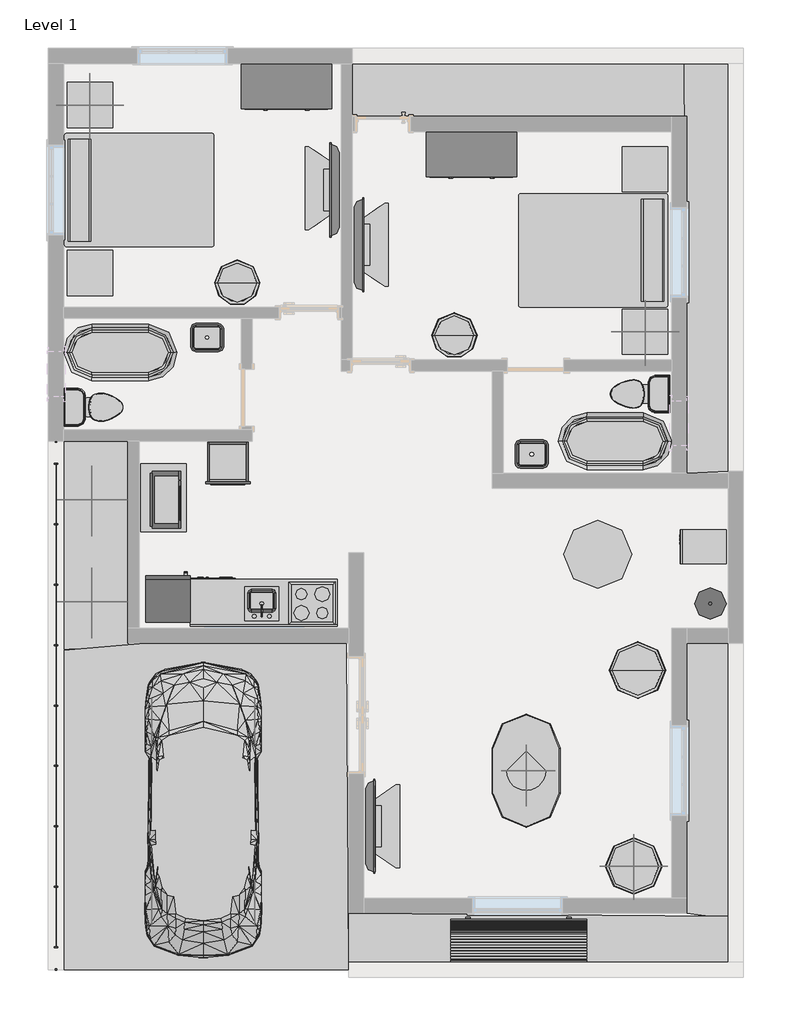
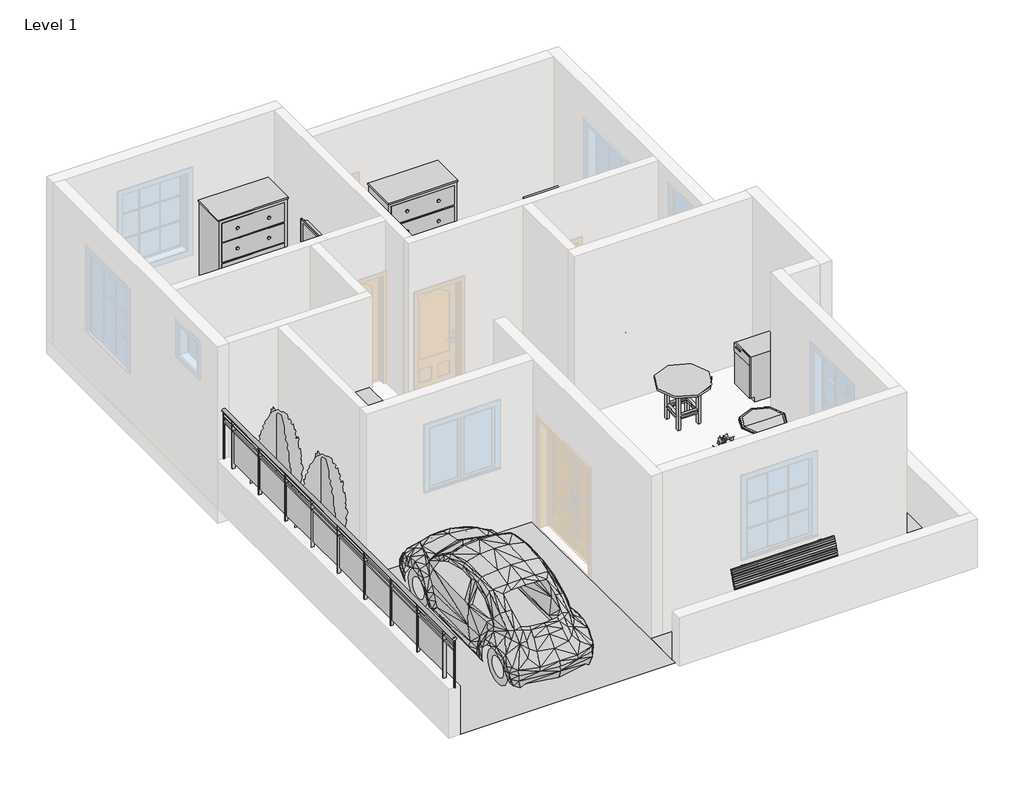
# One storey, part 2 of 2: 22 furniture elements, 14 proxies, 8 flow terminals, 7 geographic elements, 1 railing.
"""IFC4 building model written with IfcOpenShell, lengths in millimetres."""

from ifc_helpers import new_model, si_unit, point, frame, origin, place, context, project, spatial, polyline, ellipse_curve, trimmed, outline, extrude, triangles, transform, mapped, element, save
from ifc_brep_helpers import plane_surface, extruded_surface, advanced_brep
from components import proxy_7e1014cc, proxy_a6faaae8, proxy_45b28599, kitchenette_medium_kitchenette_medium_844211aa, proxy_8a8d5ab2, proxy_8b8c2dc4, rpc_beetle_rpc_beetle_3ce7ba48, proxy_c523a7b7, flow_terminal_871c2e40, flow_terminal_d49f872f, flow_terminal_62a433f7, toilet_domestic_3d_toilet_domestic_3d_f7549cf7, toilet_domestic_3d_toilet_domestic_3d_183bbd19, flow_terminal_b374fae2, furniture_e1791683, furniture_c6510c7c, furniture_9fa109b2, furniture_fdf74506, tv_stand_tv_stand_6ce107e5, furniture_582790c0, furniture_905aceb5, furniture_5bc9ed15, furniture_a672282c, table_round_2_a0cc3393, furniture_ebfaaaa6, geographic_element_235d1464, rpc_plant_tropical_55f6ff97, rpc_plant_tropical_agave_1_5_93a2a214, rpc_tree_conifer_chinese_juniper_7_1b9786cd

model = new_model("IFC4")

# Units and contexts
model_context = context("Model", 3, world=origin())
ifc_project = project(units=[si_unit("LENGTHUNIT", "METRE", prefix="MILLI")], contexts=[model_context])

# Site, building, storey
site = spatial("IfcSite", under=ifc_project)
building = spatial("IfcBuilding", under=site)
storey = spatial("IfcBuildingStorey", under=building, Name="Level 1", Elevation=0.0)

# Proxies
placement = place(None, origin())
element("IfcBuildingElementProxy", 1, Name="Building Element Proxy", at=placement, inside=storey, context=model_context, shape_type="Tessellation", body=[
    triangles([(-9901.0816956, 10267.8430298, 0.0), (-9037.4820831, 10267.8430298, 0.0), (-9037.4820831, 7550.0426422, 0.0), (-9901.0816956, 7550.0426422, 0.0), (-9901.0816956, 7466.0681168, 0.0), (-9032.7509766, 7492.9676376, 0.0), (-9033.9538101, 7484.1896851, 0.0)], [[7, 3, 5], [4, 5, 3], [1, 4, 3], [7, 6, 3], [3, 2, 1], [2, 3, 6]], closed=False),
])
element("IfcBuildingElementProxy", 2, Name="Building Element Proxy", at=placement, inside=storey, context=model_context, shape_type="Tessellation", body=[
    triangles([(-9901.0816956, 7456.8274017, 0.0), (-6098.1167313, 7550.0426422, 0.0), (-6072.0322769, 3155.8425453, 0.0), (-9901.0816956, 3155.8425453, 0.0), (-9026.5641449, 7481.0009262, 0.0), (-7567.2456619, 7524.6424484, 0.0), (-7984.5248428, 7517.1097687, 0.0), (-7982.6394928, 7524.6424484, 0.0), (-7985.2678207, 7537.342836, 0.0), (-8172.2232697, 7550.0426422, 0.0), (-8795.599173, 7550.0426422, 0.0), (-9021.7231613, 7526.2632797, 0.0)], [[4, 5, 1], [10, 5, 7], [1, 5, 12], [5, 11, 12], [11, 5, 10], [7, 9, 10], [12, 11, 1], [5, 4, 7], [8, 7, 6], [3, 7, 4], [6, 7, 3], [7, 8, 9], [6, 2, 10], [6, 9, 8], [2, 6, 3], [6, 10, 9]], closed=False),
])
element("IfcBuildingElementProxy", 3, Name="Building Element Proxy", at=placement, inside=storey, context=model_context, shape_type="Tessellation", body=[
    triangles([(-6065.6820831, 3917.8425453, 0.0), (-960.2821558, 3880.1032791, 0.0), (-960.2821558, 3257.4427391, 0.0), (-6065.6820831, 3257.4427391, 0.0)], [[1, 4, 2], [3, 2, 4]], closed=False),
])
element("IfcBuildingElementProxy", 4, Name="Building Element Proxy", at=placement, inside=storey, context=model_context, shape_type="Tessellation", body=[
    triangles([(-1519.0821316, 3917.8425453, 0.0), (-960.2821558, 3843.8738045, 0.0), (-1519.0821316, 7550.0426422, 0.0), (-960.2821558, 7550.0426422, 0.0)], [[3, 1, 4], [2, 4, 1]], closed=False),
])
element("IfcBuildingElementProxy", 5, Name="Building Element Proxy", at=placement, inside=storey, context=model_context, shape_type="Tessellation", body=[
    triangles([(-960.2821558, 9861.4422546, 0.0), (-1519.0821316, 9836.0426422, 0.0), (-1552.946925, 15347.8422546, 0.0), (-960.2821558, 15347.8422546, 0.0)], [[3, 2, 1], [1, 4, 3]], closed=False),
])
element("IfcBuildingElementProxy", 6, Name="Building Element Proxy", at=placement, inside=storey, context=model_context, shape_type="Tessellation", body=[
    triangles([(-1519.0821316, 14636.6426422, 0.0), (-1526.6161194, 15347.8422546, 0.0), (-6014.8822769, 15347.8422546, 0.0), (-6014.8822769, 14636.6426422, 0.0)], [[3, 4, 2], [1, 2, 4]], closed=False),
])
proxy_shape = proxy_7e1014cc(model_context)
element("IfcBuildingElementProxy", 7, Name="18\" x 24\" x 34 1/2\"", ObjectType="18\" x 24\" x 34 1/2\"", at=placement, inside=storey, context=model_context, shape_type="MappedRepresentation", body=[
    mapped(proxy_shape, transform((-1556.9317378, 9151.5601324, 0.0), x_axis=(0.0, -1.0000000000000004, 0.0), y_axis=(1.0000000000000004, 0.0, 0.0), z_axis=(0.0, 0.0, 1.0))),
])
proxy_2_shape = proxy_a6faaae8(model_context)
element("IfcBuildingElementProxy", 8, Name="Cook Top-4 Unit2 : 22\" x 20\"", ObjectType="Cook Top-4 Unit2 : 22\" x 20\"", at=placement, inside=storey, context=model_context, shape_type="MappedRepresentation", body=[
    mapped(proxy_2_shape, transform((-6560.982173, 8083.4426639, 0.0), x_axis=(-1.0, 0.0, 0.0), y_axis=(0.0, -1.0, 0.0), z_axis=(0.0, 0.0, 1.0))),
])
proxy_3_shape = proxy_45b28599(model_context)
element("IfcBuildingElementProxy", 9, Name="Dishwasher : 24\" x 24\" x 34\"", ObjectType="Dishwasher : 24\" x 24\" x 34\"", at=placement, inside=storey, context=model_context, shape_type="MappedRepresentation", body=[
    mapped(proxy_3_shape, transform((-7512.1647045, 8375.2922287, 0.0), x_axis=(-1.0, 0.0, 0.0), y_axis=(0.0, -1.0, 0.0), z_axis=(0.0, 0.0, 1.0))),
])
kitchenette_medium_kitchenette_medium_shape = kitchenette_medium_kitchenette_medium_844211aa(model_context)
element("IfcBuildingElementProxy", 10, Name="Kitchenette - Medium : Kitchenette - Medium", ObjectType="Kitchenette - Medium : Kitchenette - Medium", at=placement, inside=storey, context=model_context, shape_type="MappedRepresentation", body=[
    mapped(kitchenette_medium_kitchenette_medium_shape, transform((-6885.1444681, 7778.6426639, 0.0), x_axis=(-1.0, 0.0, 0.0), y_axis=(0.0, -1.0, 0.0), z_axis=(0.0, 0.0, 1.0))),
])
proxy_4_shape = proxy_8a8d5ab2(model_context)
element("IfcBuildingElementProxy", 11, Name="Microwave : 30\" x 16\" x 18\"", ObjectType="Microwave : 30\" x 16\" x 18\"", at=placement, inside=storey, context=model_context, shape_type="MappedRepresentation", body=[
    mapped(proxy_4_shape, transform((-8882.5626788, 8980.1497866, 0.0), x_axis=(0.0, 1.0, 0.0), y_axis=(-1.0, 0.0, 0.0), z_axis=(0.0, 0.0, 1.0))),
])
proxy_5_shape = proxy_8b8c2dc4(model_context)
element("IfcBuildingElementProxy", 12, Name="Oven Double-Built-in : 21 1/2\" x 39 1/4\" x 21\"", ObjectType="Oven Double-Built-in : 21 1/2\" x 39 1/4\" x 21\"", at=placement, inside=storey, context=model_context, shape_type="MappedRepresentation", body=[
    mapped(proxy_5_shape, transform((-7656.1072457, 9847.376805, 0.0), x_axis=(1.0, 0.0, 0.0), y_axis=(0.0, 1.0, 0.0), z_axis=(0.0, 0.0, 1.0))),
])
rpc_beetle_rpc_beetle_shape = rpc_beetle_rpc_beetle_3ce7ba48(model_context)
element("IfcBuildingElementProxy", 13, Name="RPC Beetle : RPC Beetle", ObjectType="RPC Beetle : RPC Beetle", at=placement, inside=storey, context=model_context, shape_type="MappedRepresentation", body=[
    mapped(rpc_beetle_rpc_beetle_shape, transform((-8021.482173, 4070.2426639, 0.0), x_axis=(1.0, 0.0, 0.0), y_axis=(0.0, 1.0, 0.0), z_axis=(0.0, 0.0, 1.0))),
])
proxy_6_shape = proxy_c523a7b7(model_context)
element("IfcBuildingElementProxy", 14, Name="Refrigerator : 24\" x 25\" LH", ObjectType="Refrigerator : 24\" x 25\" LH", at=placement, inside=storey, context=model_context, shape_type="MappedRepresentation", body=[
    mapped(proxy_6_shape, transform((-8497.732173, 8129.0916354, 0.0), x_axis=(-1.0, 0.0, 0.0), y_axis=(0.0, -1.0, 0.0), z_axis=(0.0, 0.0, 1.0))),
])

# Flow terminals
flow_terminal_shape = flow_terminal_871c2e40(model_context)
element("IfcFlowTerminal", 15, ObjectType="Sink Kitchen-Island : 18\" x 18\"", at=placement, inside=storey, context=model_context, shape_type="MappedRepresentation", body=[
    mapped(flow_terminal_shape, transform((-7218.3929324, 8085.788065, -14.4), x_axis=(-1.0, 0.0, 0.0), y_axis=(0.0, -1.0, 0.0), z_axis=(0.0, 0.0, 1.0))),
])
flow_terminal_2_shape = flow_terminal_d49f872f(model_context)
element("IfcFlowTerminal", 16, ObjectType="Sink Vanity-Round : 19\" x 19\"", at=placement, inside=storey, context=model_context, shape_type="MappedRepresentation", body=[
    mapped(flow_terminal_2_shape, transform((-1286.1174042, 8180.0944045, 609.6), x_axis=(0.0, -1.0000000000000004, 0.0), y_axis=(1.0000000000000004, 0.0, 0.0), z_axis=(0.0, 0.0, 1.0))),
])
flow_terminal_3_shape = flow_terminal_62a433f7(model_context)
element("IfcFlowTerminal", 17, ObjectType="Sink Vanity-Square : 20\" x 18\"", at=placement, inside=storey, context=model_context, shape_type="MappedRepresentation", body=[
    mapped(flow_terminal_3_shape, transform((-3586.1929324, 10041.588065, 609.6), x_axis=(-1.0, 0.0, 0.0), y_axis=(0.0, -1.0, 0.0), z_axis=(0.0, 0.0, 1.0))),
])
element("IfcFlowTerminal", 18, ObjectType="Sink Vanity-Square : 20\" x 18\"", at=placement, inside=storey, context=model_context, shape_type="MappedRepresentation", body=[
    mapped(flow_terminal_3_shape, transform((-7986.3714136, 11713.2972628, 609.6), x_axis=(0.9999999999999999, 0.0, 0.0), y_axis=(0.0, 0.9999999999999999, 0.0), z_axis=(0.0, 0.0, 1.0))),
])
toilet_domestic_3d_toilet_domestic_3d_shape = toilet_domestic_3d_toilet_domestic_3d_f7549cf7(model_context)
toilet_domestic_3d_toilet_domestic_3d_2_shape = toilet_domestic_3d_toilet_domestic_3d_183bbd19(model_context)
element("IfcFlowTerminal", 19, ObjectType="Toilet-Domestic-3D : Toilet-Domestic-3D", at=placement, inside=storey, context=model_context, shape_type="MappedRepresentation", body=[
    mapped(toilet_domestic_3d_toilet_domestic_3d_shape, transform((-9406.3861457, 10725.0426639, 0.0), x_axis=(0.0, 1.0, 0.0), y_axis=(-1.0, 0.0, 0.0), z_axis=(0.0, 0.0, 1.0))),
    mapped(toilet_domestic_3d_toilet_domestic_3d_2_shape, transform((-9406.3861457, 10725.0426639, 0.0), x_axis=(0.0, 1.0, 0.0), y_axis=(-1.0, 0.0, 0.0), z_axis=(0.0, 0.0, 1.0))),
])
element("IfcFlowTerminal", 20, ObjectType="Toilet-Domestic-3D : Toilet-Domestic-3D", at=placement, inside=storey, context=model_context, shape_type="MappedRepresentation", body=[
    mapped(toilet_domestic_3d_toilet_domestic_3d_shape, transform((-2242.3782004, 10902.8426639, 0.0), x_axis=(0.0, -1.0, 0.0), y_axis=(1.0, 0.0, 0.0), z_axis=(0.0, 0.0, 1.0))),
    mapped(toilet_domestic_3d_toilet_domestic_3d_2_shape, transform((-2242.3782004, 10902.8426639, 0.0), x_axis=(0.0, -1.0, 0.0), y_axis=(1.0, 0.0, 0.0), z_axis=(0.0, 0.0, 1.0))),
])
flow_terminal_4_shape = flow_terminal_b374fae2(model_context)
element("IfcFlowTerminal", 21, ObjectType="Tub-Free Standing-3D : 30\" x 60\"", at=placement, inside=storey, context=model_context, shape_type="MappedRepresentation", body=[
    mapped(flow_terminal_4_shape, transform((-2484.282173, 10267.8426639, 0.0), x_axis=(0.0, -1.0000000000000004, 0.0), y_axis=(1.0000000000000004, 0.0, 0.0), z_axis=(0.0, 0.0, 1.0))),
])
element("IfcFlowTerminal", 22, ObjectType="Tub-Free Standing-3D : 30\" x 60\"", at=placement, inside=storey, context=model_context, shape_type="MappedRepresentation", body=[
    mapped(flow_terminal_4_shape, transform((-9139.082173, 11461.6426639, 0.0), x_axis=(0.0, 1.0, 0.0), y_axis=(-1.0, 0.0, 0.0), z_axis=(0.0, 0.0, 1.0))),
])

# Furniture
furniture_shape = furniture_e1791683(model_context)
element("IfcFurniture", 23, ObjectType="Bed-Standard.0001 : Queen 60\" x 79\"", at=placement, inside=storey, context=model_context, shape_type="MappedRepresentation", body=[
    mapped(furniture_shape, transform((-8930.677255, 13374.5541393, 0.0), x_axis=(0.0, 1.0, 0.0), y_axis=(-1.0, 0.0, 0.0), z_axis=(0.0, 0.0, 1.0))),
])
element("IfcFurniture", 24, ObjectType="Bed-Standard.0001 : Queen 60\" x 79\"", at=placement, inside=storey, context=model_context, shape_type="MappedRepresentation", body=[
    mapped(furniture_shape, transform((-2730.787091, 13104.7311885, 0.0), x_axis=(0.0, -1.0000000000000002, 0.0), y_axis=(1.0000000000000002, 0.0, 0.0), z_axis=(0.0, 0.0, 1.0))),
])
furniture_2_shape = furniture_c6510c7c(model_context)
element("IfcFurniture", 25, ObjectType="Counter Top w Sink Hole : 24\" Depth", at=placement, inside=storey, context=model_context, shape_type="MappedRepresentation", body=[
    mapped(furniture_2_shape, transform((-7418.5444681, 7778.6426639, -14.4), x_axis=(-1.0, 0.0, 0.0), y_axis=(0.0, -1.0, 0.0), z_axis=(0.0, 0.0, 1.0))),
])
furniture_3_shape = furniture_9fa109b2(model_context)
element("IfcFurniture", 26, ObjectType="Dresser : 48\" x 72\" x 24\"", at=placement, inside=storey, context=model_context, shape_type="MappedRepresentation", body=[
    mapped(furniture_3_shape, transform((-6634.6889132, 15406.205618, 0.0), x_axis=(1.0, 0.0, 0.0), y_axis=(0.0, 1.0, 0.0), z_axis=(0.0, 0.0, 1.0))),
])
element("IfcFurniture", 27, ObjectType="Dresser : 48\" x 72\" x 24\"", at=placement, inside=storey, context=model_context, shape_type="MappedRepresentation", body=[
    mapped(furniture_3_shape, transform((-4145.4889132, 14491.805618, 0.0), x_axis=(1.0, 0.0, 0.0), y_axis=(0.0, 1.0, 0.0), z_axis=(0.0, 0.0, 1.0))),
])
furniture_4_shape = furniture_fdf74506(model_context)
element("IfcFurniture", 28, ObjectType="TV - Flat Screen : 50\"", at=placement, inside=storey, context=model_context, shape_type="MappedRepresentation", body=[
    mapped(furniture_4_shape, transform((-6251.2207967, 13642.0981498, 914.4), x_axis=(0.0, -1.0, 0.0), y_axis=(1.0, 0.0, 0.0), z_axis=(0.0, 0.0, 1.0))),
])
element("IfcFurniture", 29, ObjectType="TV - Flat Screen : 50\"", at=placement, inside=storey, context=model_context, shape_type="MappedRepresentation", body=[
    mapped(furniture_4_shape, transform((-5930.9435494, 12913.3871781, 914.4), x_axis=(0.0, 1.0000000000000002, 0.0), y_axis=(-1.0000000000000002, 0.0, 0.0), z_axis=(0.0, 0.0, 1.0))),
])
element("IfcFurniture", 30, ObjectType="TV - Flat Screen : 50\"", at=placement, inside=storey, context=model_context, shape_type="MappedRepresentation", body=[
    mapped(furniture_4_shape, transform((-5778.5435494, 5090.1871781, 914.4), x_axis=(0.0, 1.0000000000000002, 0.0), y_axis=(-1.0000000000000002, 0.0, 0.0), z_axis=(0.0, 0.0, 1.0))),
])
tv_stand_tv_stand_shape = tv_stand_tv_stand_6ce107e5(model_context)
element("IfcFurniture", 31, ObjectType="TV Stand : TV Stand", at=placement, inside=storey, context=model_context, shape_type="MappedRepresentation", body=[
    mapped(tv_stand_tv_stand_shape, transform((-6192.682173, 13796.630666, 0.0), x_axis=(0.0, -1.0, 0.0), y_axis=(1.0, 0.0, 0.0), z_axis=(0.0, 0.0, 1.0))),
])
element("IfcFurniture", 32, ObjectType="TV Stand : TV Stand", at=placement, inside=storey, context=model_context, shape_type="MappedRepresentation", body=[
    mapped(tv_stand_tv_stand_shape, transform((-5989.482173, 12784.2546618, 0.0), x_axis=(0.0, 1.0000000000000002, 0.0), y_axis=(-1.0000000000000002, 0.0, 0.0), z_axis=(0.0, 0.0, 1.0))),
])
element("IfcFurniture", 33, ObjectType="TV Stand : TV Stand", at=placement, inside=storey, context=model_context, shape_type="MappedRepresentation", body=[
    mapped(tv_stand_tv_stand_shape, transform((-5837.082173, 4961.0546618, 0.0), x_axis=(0.0, 1.0000000000000009, 0.0), y_axis=(-1.0000000000000009, 0.0, 0.0), z_axis=(0.0, 0.0, 1.0))),
])
furniture_5_shape = furniture_582790c0(model_context)
element("IfcFurniture", 34, ObjectType="Table-Dining Oval : 36\" x 72\"", at=placement, inside=storey, context=model_context, shape_type="MappedRepresentation", body=[
    mapped(furniture_5_shape, transform((-4036.1805337, 6237.362336, 0.0), x_axis=(0.0, 1.0, 0.0), y_axis=(-1.0, 0.0, 0.0), z_axis=(0.0, 0.0, 1.0))),
])
furniture_6_shape = furniture_905aceb5(model_context)
element("IfcFurniture", 35, ObjectType="Table-Dining Round w Chairs : 36\" Diameter", at=placement, inside=storey, context=model_context, shape_type="MappedRepresentation", body=[
    mapped(furniture_6_shape, transform((-2816.5641402, 8928.7213524, 0.0), x_axis=(1.0, 0.0, 0.0), y_axis=(0.0, 1.0, 0.0), z_axis=(0.0, 0.0, 1.0))),
])
furniture_7_shape = furniture_5bc9ed15(model_context)
element("IfcFurniture", 36, ObjectType="Table-Night Stand : 24\" x 24\" x 30\"", at=placement, inside=storey, context=model_context, shape_type="MappedRepresentation", body=[
    mapped(furniture_7_shape, transform((-9854.0158033, 12223.6426639, 0.0), x_axis=(1.0, 0.0, 0.0), y_axis=(0.0, 1.0, 0.0), z_axis=(0.0, 0.0, 1.0))),
])
element("IfcFurniture", 37, ObjectType="Table-Night Stand : 24\" x 24\" x 30\"", at=placement, inside=storey, context=model_context, shape_type="MappedRepresentation", body=[
    mapped(furniture_7_shape, transform((-9854.0158033, 14484.2426639, 0.0), x_axis=(1.0, 0.0, 0.0), y_axis=(0.0, 1.0, 0.0), z_axis=(0.0, 0.0, 1.0))),
])
element("IfcFurniture", 38, ObjectType="Table-Night Stand : 24\" x 24\" x 30\"", at=placement, inside=storey, context=model_context, shape_type="MappedRepresentation", body=[
    mapped(furniture_7_shape, transform((-2386.4158033, 13620.6426639, 0.0), x_axis=(1.0, 0.0, 0.0), y_axis=(0.0, 1.0, 0.0), z_axis=(0.0, 0.0, 1.0))),
])
element("IfcFurniture", 39, ObjectType="Table-Night Stand : 24\" x 24\" x 30\"", at=placement, inside=storey, context=model_context, shape_type="MappedRepresentation", body=[
    mapped(furniture_7_shape, transform((-2386.4158033, 11436.2426639, 0.0), x_axis=(1.0, 0.0, 0.0), y_axis=(0.0, 1.0, 0.0), z_axis=(0.0, 0.0, 1.0))),
])
furniture_8_shape = furniture_a672282c(model_context)
element("IfcFurniture", 40, ObjectType="Table-Rectangular : 72\" x 30\"", at=placement, inside=storey, context=model_context, shape_type="MappedRepresentation", body=[
    mapped(furniture_8_shape, transform((-8554.882173, 9505.8426639, 0.0), x_axis=(0.0, 1.0000000000000002, 0.0), y_axis=(-1.0000000000000002, 0.0, 0.0), z_axis=(0.0, 0.0, 1.0))),
])
table_round_2_shape = table_round_2_a0cc3393(model_context)
element("IfcFurniture", 41, ObjectType="Table-Round : 2", at=placement, inside=storey, context=model_context, shape_type="MappedRepresentation", body=[
    mapped(table_round_2_shape, transform((-7564.282173, 12401.4426639, 0.0), x_axis=(1.0, 0.0, 0.0), y_axis=(0.0, 1.0, 0.0), z_axis=(0.0, 0.0, 1.0))),
])
element("IfcFurniture", 42, ObjectType="Table-Round : 2", at=placement, inside=storey, context=model_context, shape_type="MappedRepresentation", body=[
    mapped(table_round_2_shape, transform((-4643.282173, 11690.2426639, 0.0), x_axis=(1.0, 0.0, 0.0), y_axis=(0.0, 1.0, 0.0), z_axis=(0.0, 0.0, 1.0))),
])
furniture_9_shape = furniture_ebfaaaa6(model_context)
element("IfcFurniture", 43, ObjectType="Table-Round : 36\" Diameter", at=placement, inside=storey, context=model_context, shape_type="MappedRepresentation", body=[
    mapped(furniture_9_shape, transform((-2230.282173, 4552.8426639, 0.0), x_axis=(1.0, 0.0, 0.0), y_axis=(0.0, 1.0, 0.0), z_axis=(0.0, 0.0, 1.0))),
])
element("IfcFurniture", 44, ObjectType="Table-Round : 36\" Diameter", at=placement, inside=storey, context=model_context, shape_type="MappedRepresentation", body=[
    mapped(furniture_9_shape, transform((-2179.482173, 7188.0926639, 0.0), x_axis=(1.0, 0.0, 0.0), y_axis=(0.0, 1.0, 0.0), z_axis=(0.0, 0.0, 1.0))),
])

# Geographic elements
geographic_element_shape = geographic_element_235d1464(model_context)
element("IfcGeographicElement", 45, ObjectType="Park Bench : 72\"", at=placement, inside=storey, context=model_context, shape_type="MappedRepresentation", body=[
    mapped(geographic_element_shape, transform((-3779.682173, 3587.6426639, 0.0), x_axis=(1.0, 0.0, 0.0), y_axis=(0.0, 1.0, 0.0), z_axis=(0.0, 0.0, 1.0))),
])
rpc_plant_tropical_shape = rpc_plant_tropical_55f6ff97(model_context)
element("IfcGeographicElement", 46, ObjectType="RPC Plant - Tropical", at=placement, inside=storey, context=model_context, shape_type="MappedRepresentation", body=[
    mapped(rpc_plant_tropical_shape, transform((-3678.082173, 5835.5426639, 914.4), x_axis=(1.0, 0.0, 0.0), y_axis=(0.0, 1.0, 0.0), z_axis=(0.0, 0.0, 1.0))),
])
rpc_plant_tropical_agave_1_5_shape = rpc_plant_tropical_agave_1_5_93a2a214(model_context)
element("IfcGeographicElement", 47, ObjectType="RPC Plant - Tropical : Agave - 1.5'", at=placement, inside=storey, context=model_context, shape_type="MappedRepresentation", body=[
    mapped(rpc_plant_tropical_agave_1_5_shape, transform((-2230.282173, 4552.8426639, 762.0), x_axis=(1.0, 0.0, 0.0), y_axis=(0.0, 1.0, 0.0), z_axis=(0.0, 0.0, 1.0))),
])
element("IfcGeographicElement", 48, ObjectType="RPC Plant - Tropical : Agave - 1.5'", at=placement, inside=storey, context=model_context, shape_type="MappedRepresentation", body=[
    mapped(rpc_plant_tropical_agave_1_5_shape, transform((-2077.882173, 11741.0426639, 762.0), x_axis=(1.0, 0.0, 0.0), y_axis=(0.0, 1.0, 0.0), z_axis=(0.0, 0.0, 1.0))),
])
element("IfcGeographicElement", 49, ObjectType="RPC Plant - Tropical : Agave - 1.5'", at=placement, inside=storey, context=model_context, shape_type="MappedRepresentation", body=[
    mapped(rpc_plant_tropical_agave_1_5_shape, transform((-9545.482173, 14789.0426639, 762.0), x_axis=(1.0, 0.0, 0.0), y_axis=(0.0, 1.0, 0.0), z_axis=(0.0, 0.0, 1.0))),
])
rpc_tree_conifer_chinese_juniper_7_shape = rpc_tree_conifer_chinese_juniper_7_1b9786cd(model_context)
element("IfcGeographicElement", 50, ObjectType="RPC Tree - Conifer : Chinese Juniper - 7'", at=placement, inside=storey, context=model_context, shape_type="MappedRepresentation", body=[
    mapped(rpc_tree_conifer_chinese_juniper_7_shape, transform((-9520.2788441, 8108.8426639, 0.0), x_axis=(1.0, 0.0, 0.0), y_axis=(0.0, 1.0, 0.0), z_axis=(0.0, 0.0, 1.0))),
])
element("IfcGeographicElement", 51, ObjectType="RPC Tree - Conifer : Chinese Juniper - 7'", at=placement, inside=storey, context=model_context, shape_type="MappedRepresentation", body=[
    mapped(rpc_tree_conifer_chinese_juniper_7_shape, transform((-9520.2788441, 9480.4426639, 0.0), x_axis=(1.0, 0.0, 0.0), y_axis=(0.0, 1.0, 0.0), z_axis=(0.0, 0.0, 1.0))),
])

# Railing
element("IfcRailing", 52, ObjectType="Glass Panel - Bottom Fill", at=placement, inside=storey, context=model_context, shape_type="SolidModel", body=[
    advanced_brep(
    [(-9964.582173, 10267.8426639, 1828.8), (-10040.782173, 10267.8426639, 1828.8), (-9964.582173, 3155.8426639, 1828.8), (-10040.782173, 3155.8426639, 1828.8)],
    [
        (0, 1, ellipse_curve(frame((-10002.682173, 10267.8426639, 1828.8), z_axis=(0.0, 1.0, 0.0), x_axis=(-1.0, 0.0, 0.0)), 38.1, 28.575)),
        (1, 0, ellipse_curve(frame((-10002.682173, 10267.8426639, 1828.8), z_axis=(0.0, 1.0, 0.0), x_axis=(-1.0, 0.0, 0.0)), 38.1, 28.575)),
        (2, 3, ellipse_curve(frame((-10002.682173, 3155.8426639, 1828.8), z_axis=(0.0, -1.0, 0.0), x_axis=(-1.0, 0.0, 0.0)), 38.1, 28.575)),
        (3, 2, ellipse_curve(frame((-10002.682173, 3155.8426639, 1828.8), z_axis=(0.0, -1.0, 0.0), x_axis=(-1.0, 0.0, 0.0)), 38.1, 28.575)),
        (0, 2),
        (3, 1),
    ],
    [
        plane_surface(frame((-10002.682173, 10267.8426639, 1828.8), z_axis=(0.0, 1.0, 0.0), x_axis=(0.0, 0.0, -1.0))),
        plane_surface(frame((-10002.682173, 3155.8426639, 1828.8), z_axis=(0.0, -1.0, 0.0), x_axis=(0.0, 0.0, -1.0))),
        extruded_surface(trimmed(ellipse_curve(frame((-10002.682173, 3155.8426639, 1828.8), z_axis=(0.0, 1.0, 0.0), x_axis=(-1.0, 0.0, 0.0)), 38.1, 28.575), [point((-9964.582173, 3155.8426639, 1828.8))], [point((-10040.782173, 3155.8426639, 1828.8))], True, "CARTESIAN"), (0.0, 7112.000000000001, 0.0), 7112.000000000001),
        extruded_surface(trimmed(ellipse_curve(frame((-10002.682173, 3155.8426639, 1828.8), z_axis=(0.0, 1.0, 0.0), x_axis=(-1.0, 0.0, 0.0)), 38.1, 28.575), [point((-10040.782173, 3155.8426639, 1828.8))], [point((-9964.582173, 3155.8426639, 1828.8))], True, "CARTESIAN"), (0.0, 7112.000000000001, 0.0), 7112.000000000001),
    ],
    [
        (0, [[1, 2]]),
        (1, [[3, 4]]),
        (2, [[-1, 5, -4, 6]]),
        (3, [[-2, -6, -3, -5]]),
    ],
),
    extrude(outline(polyline([(-10015.382173, 10267.8426639), (-9989.982173, 10267.8426639), (-9989.982173, 3155.8426639), (-10015.382173, 3155.8426639), (-10015.382173, 10267.8426639)])), frame((0.0, 0.0, 1714.5), z_axis=(0.0, 0.0, 1.0), x_axis=(1.0, 0.0, 0.0)), (0.0, 0.0, 1.0), 25.4),
    extrude(outline(polyline([(-10015.382173, 10267.8426639), (-9989.982173, 10267.8426639), (-9989.982173, 3155.8426639), (-10015.382173, 3155.8426639), (-10015.382173, 10267.8426639)])), frame((0.0, 0.0, 1612.9), z_axis=(0.0, 0.0, 1.0), x_axis=(1.0, 0.0, 0.0)), (0.0, 0.0, 1.0), 25.4),
    extrude(outline(polyline([(-10028.082173, 3466.9926639), (-9977.282173, 3466.9926639), (-9977.282173, 3454.2926639), (-10028.082173, 3454.2926639), (-10028.082173, 3466.9926639)])), frame((0.0, 0.0, 914.4), z_axis=(0.0, 0.0, 1.0), x_axis=(1.0, 0.0, 0.0)), (0.0, 0.0, 1.0), 885.6788223),
    extrude(outline(polyline([(-9996.147016, 4273.4426639), (-9996.147016, 3460.6426639), (-10002.497016, 3460.6426639), (-10002.497016, 4273.4426639), (-9996.147016, 4273.4426639)])), frame((0.0, 0.0, 1016.0), z_axis=(0.0, 0.0, 1.0), x_axis=(1.0, 0.0, 0.0)), (0.0, 0.0, 1.0), 596.9),
    extrude(outline(polyline([(-10028.082173, 4279.7926639), (-9977.282173, 4279.7926639), (-9977.282173, 4267.0926639), (-10028.082173, 4267.0926639), (-10028.082173, 4279.7926639)])), frame((0.0, 0.0, 914.4), z_axis=(0.0, 0.0, 1.0), x_axis=(1.0, 0.0, 0.0)), (0.0, 0.0, 1.0), 885.6788223),
    extrude(outline(polyline([(-9996.147016, 5086.2426639), (-9996.147016, 4273.4426639), (-10002.497016, 4273.4426639), (-10002.497016, 5086.2426639), (-9996.147016, 5086.2426639)])), frame((0.0, 0.0, 1016.0), z_axis=(0.0, 0.0, 1.0), x_axis=(1.0, 0.0, 0.0)), (0.0, 0.0, 1.0), 596.9),
    extrude(outline(polyline([(-10028.082173, 5092.5926639), (-9977.282173, 5092.5926639), (-9977.282173, 5079.8926639), (-10028.082173, 5079.8926639), (-10028.082173, 5092.5926639)])), frame((0.0, 0.0, 914.4), z_axis=(0.0, 0.0, 1.0), x_axis=(1.0, 0.0, 0.0)), (0.0, 0.0, 1.0), 885.6788223),
    extrude(outline(polyline([(-9996.147016, 5899.0426639), (-9996.147016, 5086.2426639), (-10002.497016, 5086.2426639), (-10002.497016, 5899.0426639), (-9996.147016, 5899.0426639)])), frame((0.0, 0.0, 1016.0), z_axis=(0.0, 0.0, 1.0), x_axis=(1.0, 0.0, 0.0)), (0.0, 0.0, 1.0), 596.9),
    extrude(outline(polyline([(-10028.082173, 5905.3926639), (-9977.282173, 5905.3926639), (-9977.282173, 5892.6926639), (-10028.082173, 5892.6926639), (-10028.082173, 5905.3926639)])), frame((0.0, 0.0, 914.4), z_axis=(0.0, 0.0, 1.0), x_axis=(1.0, 0.0, 0.0)), (0.0, 0.0, 1.0), 885.6788223),
    extrude(outline(polyline([(-9996.147016, 6711.8426639), (-9996.147016, 5899.0426639), (-10002.497016, 5899.0426639), (-10002.497016, 6711.8426639), (-9996.147016, 6711.8426639)])), frame((0.0, 0.0, 1016.0), z_axis=(0.0, 0.0, 1.0), x_axis=(1.0, 0.0, 0.0)), (0.0, 0.0, 1.0), 596.9),
    extrude(outline(polyline([(-10028.082173, 6718.1926639), (-9977.282173, 6718.1926639), (-9977.282173, 6705.4926639), (-10028.082173, 6705.4926639), (-10028.082173, 6718.1926639)])), frame((0.0, 0.0, 914.4), z_axis=(0.0, 0.0, 1.0), x_axis=(1.0, 0.0, 0.0)), (0.0, 0.0, 1.0), 885.6788223),
    extrude(outline(polyline([(-9996.147016, 7524.6426639), (-9996.147016, 6711.8426639), (-10002.497016, 6711.8426639), (-10002.497016, 7524.6426639), (-9996.147016, 7524.6426639)])), frame((0.0, 0.0, 1016.0), z_axis=(0.0, 0.0, 1.0), x_axis=(1.0, 0.0, 0.0)), (0.0, 0.0, 1.0), 596.9),
    extrude(outline(polyline([(-10028.082173, 7530.9926639), (-9977.282173, 7530.9926639), (-9977.282173, 7518.2926639), (-10028.082173, 7518.2926639), (-10028.082173, 7530.9926639)])), frame((0.0, 0.0, 914.4), z_axis=(0.0, 0.0, 1.0), x_axis=(1.0, 0.0, 0.0)), (0.0, 0.0, 1.0), 885.6788223),
    extrude(outline(polyline([(-9996.147016, 8337.4426639), (-9996.147016, 7524.6426639), (-10002.497016, 7524.6426639), (-10002.497016, 8337.4426639), (-9996.147016, 8337.4426639)])), frame((0.0, 0.0, 1016.0), z_axis=(0.0, 0.0, 1.0), x_axis=(1.0, 0.0, 0.0)), (0.0, 0.0, 1.0), 596.9),
    extrude(outline(polyline([(-10028.082173, 8343.7926639), (-9977.282173, 8343.7926639), (-9977.282173, 8331.0926639), (-10028.082173, 8331.0926639), (-10028.082173, 8343.7926639)])), frame((0.0, 0.0, 914.4), z_axis=(0.0, 0.0, 1.0), x_axis=(1.0, 0.0, 0.0)), (0.0, 0.0, 1.0), 885.6788223),
    extrude(outline(polyline([(-9996.147016, 9150.2426639), (-9996.147016, 8337.4426639), (-10002.497016, 8337.4426639), (-10002.497016, 9150.2426639), (-9996.147016, 9150.2426639)])), frame((0.0, 0.0, 1016.0), z_axis=(0.0, 0.0, 1.0), x_axis=(1.0, 0.0, 0.0)), (0.0, 0.0, 1.0), 596.9),
    extrude(outline(polyline([(-10028.082173, 9156.5926639), (-9977.282173, 9156.5926639), (-9977.282173, 9143.8926639), (-10028.082173, 9143.8926639), (-10028.082173, 9156.5926639)])), frame((0.0, 0.0, 914.4), z_axis=(0.0, 0.0, 1.0), x_axis=(1.0, 0.0, 0.0)), (0.0, 0.0, 1.0), 885.6788223),
    extrude(outline(polyline([(-9996.147016, 9963.0426639), (-9996.147016, 9150.2426639), (-10002.497016, 9150.2426639), (-10002.497016, 9963.0426639), (-9996.147016, 9963.0426639)])), frame((0.0, 0.0, 1016.0), z_axis=(0.0, 0.0, 1.0), x_axis=(1.0, 0.0, 0.0)), (0.0, 0.0, 1.0), 596.9),
    extrude(outline(polyline([(-10028.082173, 9969.3926639), (-9977.282173, 9969.3926639), (-9977.282173, 9956.6926639), (-10028.082173, 9956.6926639), (-10028.082173, 9969.3926639)])), frame((0.0, 0.0, 914.4), z_axis=(0.0, 0.0, 1.0), x_axis=(1.0, 0.0, 0.0)), (0.0, 0.0, 1.0), 885.6788223),
    extrude(outline(polyline([(-10012.207173, 3168.5426639), (-9993.157173, 3168.5426639), (-9993.157173, 3149.4926639), (-10012.207173, 3149.4926639), (-10012.207173, 3168.5426639)])), frame((0.0, 0.0, 914.4), z_axis=(0.0, 0.0, 1.0), x_axis=(1.0, 0.0, 0.0)), (0.0, 0.0, 1.0), 885.6788223),
    extrude(outline(polyline([(-10012.207173, 10274.1926639), (-9993.157173, 10274.1926639), (-9993.157173, 10255.1426639), (-10012.207173, 10255.1426639), (-10012.207173, 10274.1926639)])), frame((0.0, 0.0, 914.4), z_axis=(0.0, 0.0, 1.0), x_axis=(1.0, 0.0, 0.0)), (0.0, 0.0, 1.0), 885.6788223),
])

save(model, "model.ifc")

# Revit data of these elements
# Type "18\" x 24\" x 34 1/2\""
#   Label = "T"
#   Assembly Code = "E1090400"
#   Depth = 2' - 0"
#   Height = 2' - 10 1/2"
#   Width = 1' - 6"
#   Panel Face Material = Plastic, Opaque Black
#   Trach Compact. Material = Steel, Paint Finish, Ivory, Matte
#   Default Elevation = 0
# Type "Cook Top-4 Unit2 : 22\" x 20\""
#   Depth = 1' - 8"
#   Width = 1' - 10"
#   Burner Material = Steel, Chrome Plated
#   Cooktop Material = Steel, Polished
#   Default Elevation = 0
#   Assembly Code = ""
# Type "Dishwasher : 24\" x 24\" x 34\""
#   Label = "DW"
#   Assembly Code = "E1090400"
#   Depth = 2' - 0"
#   Height = 2' - 10"
#   Width = 2' - 0"
#   Dishwasher Material = Steel, Paint Finish, Ivory, Glossy
#   Panel Face Material = Plastic, Opaque Black
#   Default Elevation = 0
# Type "Kitchenette - Medium : Kitchenette - Medium"
#   Assembly Code = "E1090400"
#   Counter Length = 6' - 6"
#   Cabinet Width = 4' - 6"
#   Cabinet Height = 2' - 10 1/2"
#   Cabinet Depth = 2' - 0"
#   Toe Depth = 0' - 3"
#   Toe Height = 0' - 3 1/2"
#   Cabinet Material = Cabinets
#   Door/Drawer Material = Cabinets
#   Handle Material = Cabinets - Handles
#   Default Elevation = 0
# Type "Microwave : 30\" x 16\" x 18\""
#   Assembly Code = "E1090400"
#   Depth = 1' - 4"
#   Height = 1' - 6"
#   Width = 2' - 6"
#   Microwave Material = Laminate, Ivory, Matte
#   Default Elevation = 0
# Type "Oven Double-Built-in : 21 1/2\" x 39 1/4\" x 21\""
#   Label = "OVEN"
#   Assembly Code = "E1090400"
#   Depth = 1' - 9"
#   Height = 3' - 3 1/4"
#   Width = 1' - 9 1/2"
#   Oven Material = Metal - Stainless Steel, Polished
#   Default Elevation = 0
# Type "RPC Beetle : RPC Beetle"
#   built-in parameter 1005195 = "RPC-16-0U6E-L4EG-ENH1-J3KF-SVEL-0TX4-C0"
#   Height = 0
# Type "Refrigerator : 24\" x 25\" LH"
#   Label = "REF."
#   Assembly Code = "E1090400"
#   Depth = 2' - 0 3/4"
#   Handle = 0' - 1 1/2"
#   Height = 5' - 3 1/2"
#   Rear Clearance = 0' - 2"
#   Top Door Height = 1' - 8"
#   Width = 1' - 11 1/2"
#   Material = Steel, Paint Finish, Ivory, Glossy
#   Default Elevation = 0
# Type "Sink Kitchen-Island : 18\" x 18\""
#   Assembly Code = "D2010410"
#   Counter Height = 3' - 0"
#   Depth = 1' - 6"
#   Width = 1' - 6"
#   Faucet Material = Steel, Polished
#   Sink Material = Steel, Polished
#   Default Elevation = 0
# Type "Sink Vanity-Round : 19\" x 19\""
#   Assembly Code = "D2010400"
#   Top Of Counter = 2' - 7"
#   Basin Material = Porcelain, Linen
#   Faucet Material = Steel, Polished
#   Default Elevation = 0
# Type "Sink Vanity-Square : 20\" x 18\""
#   Assembly Code = "D2010400"
#   Counter Height = 2' - 7"
#   Depth = 1' - 6"
#   Width = 1' - 8"
#   Basin Material = Porcelain, Linen
#   Faucet Material = Steel, Polished
#   Default Elevation = 0
# Type "Toilet-Domestic-3D : Toilet-Domestic-3D"
#   Assembly Code = "D2010110"
#   Toilet - Bowl/Basin Material = Porcelain, Linen
#   Toilet - Seat Material = Laminate, Linen, Matte
#   Default Elevation = 0
# Type "Tub-Free Standing-3D : 30\" x 60\""
#   Assembly Code = "D2010110"
#   Height = 1' - 6"
#   Length = 5' - 0"
#   Width = 2' - 6"
#   Tub Material = Porcelain, Ivory
#   Default Elevation = 0
# Type "Bed-Standard.0001 : Queen 60\" x 79\""
#   Assembly Code = "E2020200"
#   Length = 6' - 7"
#   Width = 5' - 0"
#   Leg Material = Steel, Chrome Plated
#   Mattress Material = Linen, White
#   Default Elevation = 0
# Type "Counter Top w Sink Hole : 24\" Depth"
#   Assembly Code = "C1030400"
#   Counter Thickness = 0' - 1 1/2"
#   Depth [instance default] = 2' - 1"
#   Height = 3' - 0"
#   Length [instance default] = 8' - 0"
#   Sink Location [instance default] = 2' - 0"
#   Sink Location To Wall [instance default] = 0' - 6"
#   Sink Opening Depth [instance default] = 1' - 3"
#   Sink Opening Width [instance default] = 2' - 3"
#   Counter Top Material = none
#   Default Elevation = 0
# Type "Dresser : 48\" x 72\" x 24\""
#   Assembly Code = "E2020200"
#   Depth = 2' - 0"
#   Height = 6' - 0"
#   Width = 4' - 0"
#   Dresser Material = Laminate - Ivory, Glossy
#   Drawer Material = Laminate, Ivory, Matte
#   Knob Material = Cherry
#   Default Elevation = 0
# Type "TV - Flat Screen : 50\""
#   SinAng = 0' - 0.0193"
#   L = 3' - 7.57782"
#   H = 2' - 0.51477"
#   Thickness = 0' - 4.33071"
#   Diagonal = 4' - 2"
#   CosAng = 0' - 0.03431"
#   Stand [instance default] = yes
#   Default Elevation = 0
# Type "TV Stand : TV Stand"
#   Depth = 1' - 6"
#   Width = 3' - 8"
#   Height = 1' - 7 1/2"
#   Finish = Melamine - Gray
#   Default Elevation = 0
# Type "Table-Dining Oval : 36\" x 72\""
#   Assembly Code = "E2020200"
#   Length = 5' - 0"
#   Width = 3' - 0"
#   Base Material = Steel, Chrome Plated
#   Top Material = Glass - Clear, Grey
#   Default Elevation = 0
#   Description = (empty or 0)
# Type "Table-Dining Round w Chairs : 36\" Diameter"
#   Assembly Code = "E2020200"
#   Radius = 1' - 6"
#   Diameter = 3' - 0"
#   Height = 2' - 6"
#   Chairs = 4
#   Base Material = Pine
#   Top Material = Laminate, Linen, Matte
#   Default Elevation = 0
# Type "Table-Night Stand : 24\" x 24\" x 30\""
#   Assembly Code = "E2020200"
#   Depth = 2' - 0"
#   Height = 2' - 6"
#   Width = 2' - 0"
#   Base Material = Birch
#   Top Material = Laminate, Ivory, Matte
#   Default Elevation = 0
# Type "Table-Rectangular : 72\" x 30\""
#   Assembly Code = "E2020200"
#   Height = 2' - 6"
#   Length = 3' - 0"
#   Width = 2' - 0"
#   Base Material = Birch
#   Top Material = Birch
#   Default Elevation = 0
# Type "Table-Round : 2"
#   Assembly Code = "E2020200"
#   Base Radius = 0' - 10"
#   Height = 2' - 6"
#   Radius = 1' - 0"
#   Base Material = Steel, Chrome Plated
#   Top Material = Birch
#   Default Elevation = 0
# Type "Table-Round : 36\" Diameter"
#   Assembly Code = "E2020200"
#   Base Radius = 0' - 10"
#   Height = 2' - 6"
#   Radius = 1' - 3"
#   Base Material = Steel, Chrome Plated
#   Top Material = Birch
#   Default Elevation = 0
# Type "Park Bench : 72\""
#   Length = 6' - 0"
#   Seat Material = Wood - Teak
#   Frame Material = Steel, Paint Finish, Dark Gray, Matte
# Type "RPC Plant - Tropical"
#   built-in parameter 1005198 = "{2, 15},{39, RPC-16-FWM5-GM7X-C67P-4000-ST1L-LVER-AU},{1, 0},{1, 0},{2, 13},{1, 8},{5, Color},{1, 0},{1, 0},{3, 0.8},{3, 0.8},{3, 0.8},{1, 8},{7, BBoxMin},{1, 0},{1, 0},{1, 0},{1, 0},{1, 0},{1, 8},{7, BBoxMax},{1, 0},{1, 0},{1, 0},{1, 0},{1, 0},{2, 11},{9, RPCTypeId},{1, 0},{1, 0},{39, RPC-16-FWM5-GM7X-C67P-4000-ST1L-LVER-AU},{1, 6},{14, RPCPlantHeight},{1, 0},{1, 0},{1, 3},{2, 11},{7, keyword},{1, 0},{1, 0},{35, :RPCs:Shrubs [General]:Geometry:RPC},{2, 11},{8, category},{1, 0},{1, 0},{16, Shrubs [General]},{2, 11},{12, LocalizedUID},{1, 0},{1, 0},{10, Crane Lily},{2, 14},{6, Height},{1, 0},{1, 0},{1, 3},{1, 2},{16, Cast Reflections},{1, 0},{1, 0},{1, 0},{1, 2},{12, Cast Shadows},{1, 0},{1, 0},{1, 1},{1, 2},{9, Lock View},{1, 0},{1, 0},{1, 0},{1, 4},{5, ViewC},{1, 0},{1, 0},{1, 0},{21, assetlibrary_base.fbx},{1, 5},"
#   built-in parameter 1005195 = "RPC-16-FWM5-GM7X-C67P-4000-ST1L-LVER-AU"
#   Assembly Code = "G2050500"
#   Height = 3' - 0"
#   Default Elevation = 0
# Type "RPC Plant - Tropical : Agave - 1.5'"
#   built-in parameter 1005198 = "{2, 15},{39, RPC-16-G1GJ-63FX-7K5P-N000-ST1L-LVER-AU},{1, 0},{1, 0},{2, 13},{1, 8},{5, Color},{1, 0},{1, 0},{3, 0.8},{3, 0.8},{3, 0.8},{1, 8},{7, BBoxMin},{1, 0},{1, 0},{1, 0},{1, 0},{1, 0},{1, 8},{7, BBoxMax},{1, 0},{1, 0},{1, 0},{1, 0},{1, 0},{2, 11},{9, RPCTypeId},{1, 0},{1, 0},{39, RPC-16-G1GJ-63FX-7K5P-N000-ST1L-LVER-AU},{1, 6},{14, RPCPlantHeight},{1, 0},{1, 0},{3, 1.5},{2, 11},{7, keyword},{1, 0},{1, 0},{35, :RPCs:Plants [General]:Geometry:RPC},{2, 11},{8, category},{1, 0},{1, 0},{16, Plants [General]},{2, 11},{12, LocalizedUID},{1, 0},{1, 0},{5, Agave},{2, 14},{6, Height},{1, 0},{1, 0},{3, 1.5},{1, 2},{16, Cast Reflections},{1, 0},{1, 0},{1, 0},{1, 2},{12, Cast Shadows},{1, 0},{1, 0},{1, 1},{1, 2},{9, Lock View},{1, 0},{1, 0},{1, 0},{1, 4},{5, ViewC},{1, 0},{1, 0},{1, 0},{21, assetlibrary_base.fbx},{1, 5},"
#   built-in parameter 1005195 = "RPC-16-G1GJ-63FX-7K5P-N000-ST1L-LVER-AU"
#   Type Comments = "Agave"
#   Assembly Code = "G2050500"
#   Height = 1' - 6"
#   Default Elevation = 0
# Type "RPC Tree - Conifer : Chinese Juniper - 7'"
#   built-in parameter 1005198 = "{2, 15},{39, RPC-16-FUM3-UUQ0-UBF0-N000-ST1L-LVER-AU},{1, 0},{1, 0},{2, 13},{1, 8},{5, Color},{1, 0},{1, 0},{3, 0.8},{3, 0.8},{3, 0.8},{1, 8},{7, BBoxMin},{1, 0},{1, 0},{1, 0},{1, 0},{1, 0},{1, 8},{7, BBoxMax},{1, 0},{1, 0},{1, 0},{1, 0},{1, 0},{2, 11},{9, RPCTypeId},{1, 0},{1, 0},{39, RPC-16-FUM3-UUQ0-UBF0-N000-ST1L-LVER-AU},{1, 6},{14, RPCPlantHeight},{1, 0},{1, 0},{1, 7},{2, 11},{7, keyword},{1, 0},{1, 0},{34, :RPCs:Trees [General]:Geometry:RPC},{2, 11},{8, category},{1, 0},{1, 0},{15, Trees [General]},{2, 11},{12, LocalizedUID},{1, 0},{1, 0},{15, Chinese Juniper},{2, 14},{6, Height},{1, 0},{1, 0},{1, 7},{1, 2},{16, Cast Reflections},{1, 0},{1, 0},{1, 0},{1, 2},{12, Cast Shadows},{1, 0},{1, 0},{1, 1},{1, 2},{9, Lock View},{1, 0},{1, 0},{1, 0},{1, 4},{5, ViewC},{1, 0},{1, 0},{1, 0},{21, assetlibrary_base.fbx},{1, 5},"
#   built-in parameter 1005195 = "RPC-16-FUM3-UUQ0-UBF0-N000-ST1L-LVER-AU"
#   Type Comments = "Chinese Juniper"
#   Assembly Code = "G2050500"
#   Height = 7' - 0"
#   Description = (empty or 0)
#   Default Elevation = 0
# Type "Glass Panel - Bottom Fill"
#   Assembly Code = "C2010400"
#   built-in parameter 1008612 = 0.0416667 (stored number, unit not read)
#   built-in parameter 1008611 = 0.0416667 (stored number, unit not read)
#   built-in parameter 1008609 = 0.333333 (stored number, unit not read)
#   built-in parameter 1008604 = 0.166667 (stored number, unit not read)
#   built-in parameter 1008603 = 0.166667 (stored number, unit not read)
#   Railing Height = 3' - 0"
#   built-in parameter 1008630 = 2
#   built-in parameter 1008610 = 2
#   built-in parameter 1008618 = Baluster - Square : 3/4"
# Element 1 (IfcBuildingElementProxy)
#   Material = Default Mass Floor
#   Phase Created = New Construction
# Elements 2, 3, 4, 5, 6 (IfcBuildingElementProxy)
#   Material = none
#   Phase Created = New Construction
# Element 7 (IfcBuildingElementProxy, "18\" x 24\" x 34 1/2\"")
#   Phase Created = New Construction
#   Materials on its faces: "Steel, Paint Finish, Ivory, Matte", "Plastic, Opaque Black"
# Element 8 (IfcBuildingElementProxy, "Cook Top-4 Unit2 : 22\" x 20\"")
#   Phase Created = New Construction
#   Materials on its faces: "Steel, Chrome Plated", "Steel, Polished"
# Element 9 (IfcBuildingElementProxy, "Dishwasher : 24\" x 24\" x 34\"")
#   Phase Created = New Construction
#   Materials on its faces: "Steel, Paint Finish, Ivory, Glossy", "Plastic, Opaque Black"
# Element 10 (IfcBuildingElementProxy, "Kitchenette - Medium : Kitchenette - Medium")
#   Phase Created = New Construction
#   Materials on its faces: "Cabinets", "Cabinets - Handles"
# Element 11 (IfcBuildingElementProxy, "Microwave : 30\" x 16\" x 18\"")
#   Phase Created = New Construction
#   Materials on its faces: "Laminate, Ivory, Matte", "Glass"
# Element 12 (IfcBuildingElementProxy, "Oven Double-Built-in : 21 1/2\" x 39 1/4\" x 21\"")
#   Phase Created = New Construction
#   Materials on its faces: "Steel", "Metal - Stainless Steel, Polished", "Glass"
# Element 13 (IfcBuildingElementProxy, "RPC Beetle : RPC Beetle")
#   Phase Created = New Construction
# Element 14 (IfcBuildingElementProxy, "Refrigerator : 24\" x 25\" LH")
#   Phase Created = New Construction
#   Materials on its faces: "Steel, Paint Finish, Ivory, Glossy", "Steel, Chrome Plated"
# Element 15 (IfcFlowTerminal, "Sink Kitchen-Island : 18\" x 18\"")
#   Mark = "7"
#   Phase Created = New Construction
#   Materials on its faces: "Steel, Polished"
# Element 16 (IfcFlowTerminal, "Sink Vanity-Round : 19\" x 19\"")
#   Mark = "8"
#   Phase Created = New Construction
#   Materials on its faces: "Porcelain, Linen", "Steel, Polished"
# Element 17 (IfcFlowTerminal, "Sink Vanity-Square : 20\" x 18\"")
#   Mark = "5"
#   Phase Created = New Construction
#   Materials on its faces: "Porcelain, Linen", "Steel, Polished"
# Element 18 (IfcFlowTerminal, "Sink Vanity-Square : 20\" x 18\"")
#   Mark = "6"
#   Phase Created = New Construction
#   Materials on its faces: "Porcelain, Linen", "Steel, Polished"
# Element 19 (IfcFlowTerminal, "Toilet-Domestic-3D : Toilet-Domestic-3D")
#   Mark = "1"
#   Phase Created = New Construction
#   Materials on its faces: "Porcelain, Linen", "Laminate, Linen, Matte"
# Element 20 (IfcFlowTerminal, "Toilet-Domestic-3D : Toilet-Domestic-3D")
#   Mark = "2"
#   Phase Created = New Construction
#   Materials on its faces: "Porcelain, Linen", "Laminate, Linen, Matte"
# Element 21 (IfcFlowTerminal, "Tub-Free Standing-3D : 30\" x 60\"")
#   Mark = "3"
#   Phase Created = New Construction
#   Materials on its faces: "Porcelain, Ivory"
# Element 22 (IfcFlowTerminal, "Tub-Free Standing-3D : 30\" x 60\"")
#   Mark = "4"
#   Phase Created = New Construction
#   Materials on its faces: "Porcelain, Ivory"
# Elements 23, 24 (IfcFurniture, "Bed-Standard.0001 : Queen 60\" x 79\"")
#   Phase Created = New Construction
#   Materials on its faces: "Linen, White", "Steel, Chrome Plated"
# Element 25 (IfcFurniture, "Counter Top w Sink Hole : 24\" Depth")
#   Sink Opening Depth = 1' - 2"
#   Sink Location To Wall = 0' - 6"
#   Length = 6' - 6"
#   Sink Location = 3' - 4"
#   Sink Opening Width = 1' - 4"
#   Depth = 2' - 1"
#   Phase Created = New Construction
#   Materials on its faces: "Counter Top"
# Elements 26, 27 (IfcFurniture, "Dresser : 48\" x 72\" x 24\"")
#   Phase Created = New Construction
#   Materials on its faces: "Laminate, Ivory, Matte", "Cherry", "Laminate - Ivory, Glossy"
# Elements 28, 29, 30 (IfcFurniture, "TV - Flat Screen : 50\"")
#   Stand = yes
#   Phase Created = New Construction
#   Materials on its faces: "TV - Black", "TV - Glass", "TV - Screen"
# Elements 31, 32, 33 (IfcFurniture, "TV Stand : TV Stand")
#   Phase Created = New Construction
#   Materials on its faces: "Melamine - Gray", "Glass - Shelves"
# Element 34 (IfcFurniture, "Table-Dining Oval : 36\" x 72\"")
#   Phase Created = New Construction
#   Materials on its faces: "Steel, Chrome Plated", "Glass - Clear, Grey"
# Element 35 (IfcFurniture, "Table-Dining Round w Chairs : 36\" Diameter")
#   Phase Created = New Construction
#   Materials on its faces: "Pine", "Laminate, Linen, Matte"
# Elements 36, 37, 38, 39 (IfcFurniture, "Table-Night Stand : 24\" x 24\" x 30\"")
#   Phase Created = New Construction
#   Materials on its faces: "Birch", "Laminate, Ivory, Matte"
# Element 40 (IfcFurniture, "Table-Rectangular : 72\" x 30\"")
#   Phase Created = New Construction
#   Materials on its faces: "Birch"
# Elements 41, 42 (IfcFurniture, "Table-Round : 2")
#   Phase Created = New Construction
#   Materials on its faces: "Steel, Chrome Plated", "Birch"
# Elements 43, 44 (IfcFurniture, "Table-Round : 36\" Diameter")
#   Phase Created = New Construction
#   Materials on its faces: "Steel, Chrome Plated", "Birch"
# Element 45 (IfcGeographicElement, "Park Bench : 72\"")
#   Phase Created = New Construction
#   Materials on its faces: "Wood - Teak", "Steel, Paint Finish, Dark Gray, Matte"
# Element 46 (IfcGeographicElement, "RPC Plant - Tropical")
#   Phase Created = New Construction
# Elements 47, 48, 49 (IfcGeographicElement, "RPC Plant - Tropical : Agave - 1.5'")
#   Phase Created = New Construction
# Elements 50, 51 (IfcGeographicElement, "RPC Tree - Conifer : Chinese Juniper - 7'")
#   Phase Created = New Construction
# Element 52 (IfcRailing, "Glass Panel - Bottom Fill")
#   built-in parameter 1008621 = 3 (stored number, unit not read)
#   Phase Created = New Construction
#   Materials on its faces: "Glass"
# Materials
#   "Plastic, Opaque Black": class "Plastic", colour RGB 0 0 0, transparency 0.7, Description = "Plastic, generic, opaque black", Cost = 0
#   "Steel, Paint Finish, Ivory, Matte": class "Metal", colour RGB 247 247 239, transparency 0, Description = "Steel, paint finish, ivory, matte", Cost = 0
#   "Steel, Chrome Plated": class "Metal", colour RGB 17 17 17, transparency 0, Description = "Chromiuim plated steel", Cost = 0
#   "Steel, Polished": class "Metal", colour RGB 57 57 57, transparency 0, Description = "Polished steel", Cost = 0
#   "Steel, Paint Finish, Ivory, Glossy": class "Metal", colour RGB 247 247 239, transparency 0, Description = "Steel, paint finish, ivory, glossy", Cost = 0
#   "Cabinets": colour RGB 249 249 249, transparency 0
#   "Cabinets - Handles": class "Metal", colour RGB 57 57 57, transparency 0
#   "Laminate, Ivory, Matte": class "Plastic", colour RGB 247 247 239, transparency 0, Description = "Plastic Laminate - Ivory, Matte", Cost = 0
#   "Metal - Stainless Steel, Polished": class "Metal", colour RGB 216 216 216, transparency 0
#   "Porcelain, Linen": class "Ceramic", colour RGB 249 239 230, transparency 0, Description = "Porcelain, linen", Cost = 0
#   "Laminate, Linen, Matte": class "Plastic", colour RGB 249 239 230, transparency 0, Description = "Plastic Laminate - Linen, Matte", Cost = 0
#   "Porcelain, Ivory": class "Ceramic", colour RGB 247 247 239, transparency 0, Description = "Porcelain, ivory", Cost = 0
#   "Linen, White": class "Textile", colour RGB 247 247 239, transparency 0, Description = "Linen, white", Cost = 0
#   "Laminate - Ivory, Glossy": colour RGB 247 247 239, transparency 0
#   "Cherry": class "Wood", colour RGB 226 177 128, transparency 0, Description = "Prunus Serotina", Cost = 0
#   "Melamine - Gray": class "Wood", colour RGB 49 49 49, transparency 0
#   "Glass - Clear, Grey": class "Glass", colour RGB 252 255 255, transparency 0.64
#   "Pine": class "Wood", colour RGB 223 192 134, transparency 0, Description = "Pinus Echinata", Cost = 0
#   "Birch": class "Wood", colour RGB 224 178 126, transparency 0, Description = "Betula Alleghaniensis", Cost = 0
#   "Wood - Teak": class "Wood", colour RGB 120 73 19, transparency 0
#   "Steel, Paint Finish, Dark Gray, Matte": class "Metal", colour RGB 98 98 98, transparency 0, Description = "Steel, paint finish, dark gray, matte", Cost = 0
#   "Default Mass Floor": colour RGB 0 255 0, transparency 0, Cost = 0
#   "Glass": class "Glass", colour RGB 0 128 192, transparency 0.75, Description = "Soda Lime Glass", Cost = 0
#   "Steel": class "Metal", colour RGB 247 247 247, transparency 0, Description = "Steel, mill finish", Cost = 0
#   "Counter Top": class "Wood", colour RGB 226 177 128, transparency 0
#   "TV - Black": colour RGB 49 49 49, transparency 0
#   "TV - Glass": colour RGB 157 157 157, transparency 0.9
#   "TV - Screen": colour RGB 0 0 0, transparency 0
#   "Glass - Shelves": class "Glass", colour RGB 167 167 167, transparency 0.9
